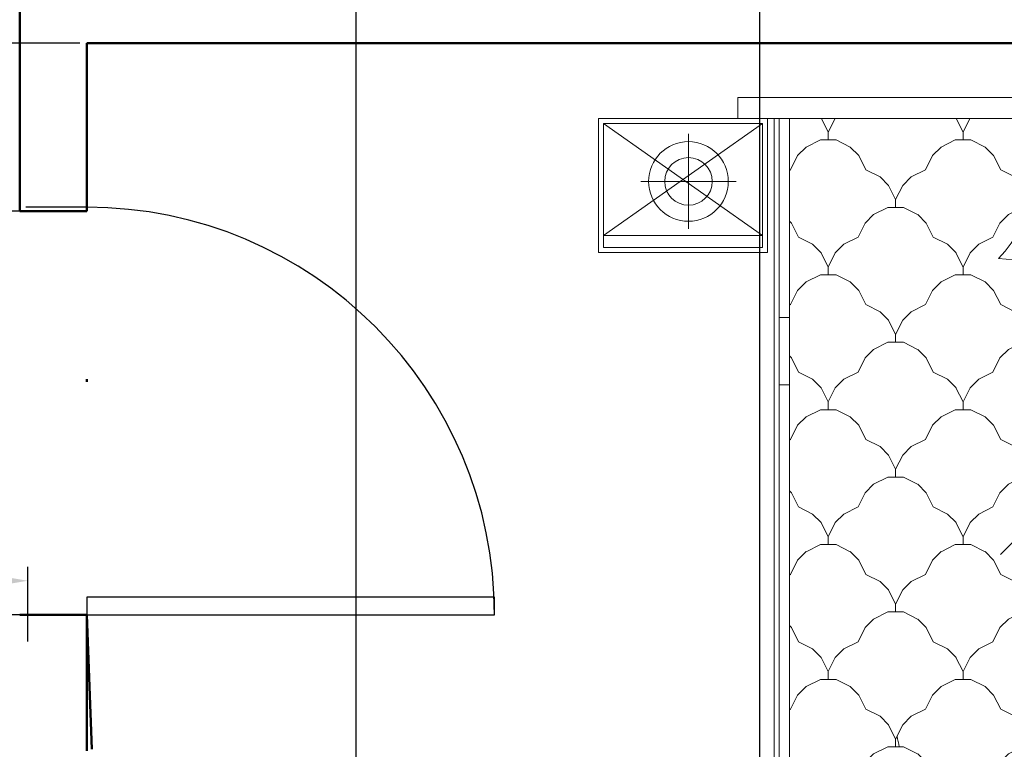
# Model space of a CAD drawing. Units: inches. Extents: x 2385 to 2740, y 1752 to 2305.
# Tile 4 of 15: x 2553 to 2641, y 1916 to 1981. Entities that reach past the tile are written whole.
import ezdxf

# ---------------------------------------------------------------- set-up
doc = ezdxf.new("R2010")
doc.units = ezdxf.units.IN
for name, color, linetype, lineweight in [('A-ANNO-DIMS', 2, 'Continuous', 18), ('A-DOOR', 4, 'Continuous', 25), ('A-FURN', 9, 'Continuous', 18), ('A-WALL', 7, 'Continuous', 50)]:
    doc.layers.add(name, color=color, linetype=linetype, lineweight=lineweight)
doc.styles.get("Standard").update_dxf_attribs({"font": 'arial.ttf'})
doc.dimstyles.new('Copy of ISO-25', dxfattribs={"dimtxt": 2.5, "dimasz": 2.5, "dimexe": 1.25, "dimexo": 0.625, "dimtad": 1, "dimdec": 1, "dimlunit": 4, "dimtxsty": 'Standard', "dimcen": 2.5, "dimadec": 0, "dimazin": 0, "dimtfac": 1, "dimtdec": 1, "dimtmove": 0, "dimatfit": 3, "dimfxl": 1, "dimarcsym": 0})

# ---------------------------------------------------------------- blocks, each defined once
blk = doc.blocks.new('A$C029D5C69')
for p, q in [((0.4164, 2.0693), (0.4164, 2.0066)), ((2.2315, 2.0693), (0.4164, 2.0693)), ((2.2315, 2.0066), (2.2315, 2.0693)), ((0, 1.606), (0, 2.0066)), ((0, 2.0066), (0.505, 2.0066)), ((0.4164, 2.0066), (2.2315, 2.0066)), ((0.505, 2.0066), (0.505, 1.606)), ((0.5252, 0.0351), (0.5252, 2.0066)), ((0.5403, 0.0502), (0.5403, 2.0066)), ((0.5706, 0.0805), (0.5706, 2.0066)), ((0.6869, 1.966), (0.6666, 2.0066)), ((0.7072, 2.0066), (0.6869, 1.966)), ((1.0902, 1.966), (1.0699, 2.0066)), ((1.1106, 2.0066), (1.0902, 1.966)), ((2.1114, 2.0087), (2.1114, 0.0351)), ((2.6479, 2.0066), (2.1429, 2.0066)), ((2.1429, 2.0066), (2.1429, 1.606)), ((2.6479, 1.606), (2.6479, 2.0066)), ((0.0151, 1.6211), (0.0151, 1.9915)), ((0.0151, 1.9915), (0.4899, 1.9915)), ((0.4899, 1.9915), (0.4899, 1.6211)), ((1.8954, 1.9865), (1.3081, 1.9865)), ((2.6328, 1.9915), (2.158, 1.9915)), ((2.158, 1.9915), (2.158, 1.6211)), ((2.6328, 1.6211), (2.6328, 1.9915)), ((0.2689, 1.9609), (0.2689, 1.6764)), ((0.6869, 1.9425), (0.6869, 1.966)), ((0.6869, 1.9425), (0.6869, 1.966)), ((1.0902, 1.9425), (1.0902, 1.966)), ((1.0902, 1.9425), (1.0902, 1.966)), ((1.8954, 1.9713), (1.3339, 1.9713)), ((1.3849, 1.9713), (1.3656, 1.952)), ((1.3945, 1.9713), (1.3714, 1.9483)), ((1.4249, 1.945), (1.3986, 1.9713)), ((1.4249, 1.945), (1.4059, 1.926)), ((1.4288, 1.9507), (1.4081, 1.9713)), ((1.4476, 1.9507), (1.4288, 1.9507)), ((1.4476, 1.9507), (1.4664, 1.9507)), ((1.487, 1.9713), (1.4664, 1.9507)), ((1.4966, 1.9713), (1.4703, 1.945)), ((1.4986, 1.9167), (1.4703, 1.945)), ((1.527, 1.945), (1.4986, 1.9167)), ((1.527, 1.945), (1.5007, 1.9713)), ((1.5309, 1.9507), (1.5102, 1.9713)), ((1.5497, 1.9507), (1.5309, 1.9507)), ((1.5497, 1.9507), (1.5685, 1.9507)), ((1.5891, 1.9713), (1.5685, 1.9507)), ((1.5987, 1.9713), (1.5724, 1.945)), ((1.6007, 1.9167), (1.5724, 1.945)), ((1.6291, 1.945), (1.6007, 1.9167)), ((1.6291, 1.945), (1.6028, 1.9713)), ((1.633, 1.9507), (1.6123, 1.9713)), ((1.6518, 1.9507), (1.633, 1.9507)), ((1.6518, 1.9507), (1.6706, 1.9507)), ((1.6912, 1.9713), (1.6706, 1.9507)), ((1.7008, 1.9713), (1.6745, 1.945)), ((1.7028, 1.9167), (1.6745, 1.945)), ((1.7312, 1.945), (1.7028, 1.9167)), ((1.7312, 1.945), (1.7049, 1.9713)), ((1.7351, 1.9507), (1.7144, 1.9713)), ((1.7539, 1.9507), (1.7351, 1.9507)), ((1.7539, 1.9507), (1.7727, 1.9507)), ((1.7933, 1.9713), (1.7727, 1.9507)), ((1.8029, 1.9713), (1.7766, 1.945)), ((1.8049, 1.9167), (1.7766, 1.945)), ((1.8333, 1.945), (1.8049, 1.9167)), ((1.8333, 1.945), (1.807, 1.9713)), ((1.8372, 1.9507), (1.8165, 1.9713)), ((1.856, 1.9507), (1.8372, 1.9507)), ((1.856, 1.9507), (1.8748, 1.9507)), ((1.8954, 1.9713), (1.8748, 1.9507)), ((1.9043, 1.9707), (1.8787, 1.945)), ((1.907, 1.9167), (1.8787, 1.945)), ((1.9354, 1.945), (1.907, 1.9167)), ((1.9354, 1.945), (1.9114, 1.969)), ((2.379, 1.9609), (2.379, 1.6764)), ((0.621, 1.9213), (0.5955, 1.8958)), ((0.6634, 1.9425), (0.621, 1.9213)), ((0.6634, 1.9425), (0.621, 1.9213)), ((0.6869, 1.9425), (0.6634, 1.9425)), ((0.6869, 1.9425), (0.7104, 1.9425)), ((0.7528, 1.9213), (0.7104, 1.9425)), ((0.7528, 1.9213), (0.7104, 1.9425)), ((0.7783, 1.8958), (0.7528, 1.9213)), ((1.0243, 1.9213), (0.9988, 1.8958)), ((1.0668, 1.9425), (1.0244, 1.9213)), ((1.0668, 1.9425), (1.0244, 1.9213)), ((1.0902, 1.9425), (1.0668, 1.9425)), ((1.0902, 1.9425), (1.1137, 1.9425)), ((1.1561, 1.9213), (1.1137, 1.9425)), ((1.1561, 1.9213), (1.1137, 1.9425)), ((1.1816, 1.8958), (1.1561, 1.9213)), ((1.4288, 1.9394), (1.4116, 1.9222)), ((1.4288, 1.9393), (1.4476, 1.9393)), ((1.4664, 1.9393), (1.4476, 1.9393)), ((1.493, 1.9128), (1.4664, 1.9394)), ((1.5309, 1.9394), (1.5043, 1.9128)), ((1.5309, 1.9393), (1.5497, 1.9393)), ((1.5685, 1.9393), (1.5497, 1.9393)), ((1.595, 1.9128), (1.5685, 1.9394)), ((1.633, 1.9394), (1.6064, 1.9128)), ((1.633, 1.9393), (1.6518, 1.9393)), ((1.6706, 1.9393), (1.6518, 1.9393)), ((1.6971, 1.9128), (1.6706, 1.9394)), ((1.7351, 1.9394), (1.7085, 1.9128)), ((1.7351, 1.9393), (1.7539, 1.9393)), ((1.7727, 1.9393), (1.7539, 1.9393)), ((1.7992, 1.9128), (1.7727, 1.9394)), ((1.8372, 1.9394), (1.8106, 1.9128)), ((1.8372, 1.9393), (1.856, 1.9393)), ((1.8748, 1.9393), (1.856, 1.9393)), ((1.9013, 1.9128), (1.8748, 1.9394)), ((1.9393, 1.9394), (1.9127, 1.9128)), ((1.9393, 1.9393), (1.9404, 1.9393)), ((1.9414, 1.688), (1.9414, 1.931)), ((1.9565, 1.688), (1.9565, 1.931)), ((0.5955, 1.8958), (0.5743, 1.8534)), ((0.7995, 1.8534), (0.7783, 1.8958)), ((0.9989, 1.8958), (0.9777, 1.8534)), ((1.2028, 1.8534), (1.1816, 1.8958)), ((1.493, 1.8752), (1.493, 1.9128)), ((1.5043, 1.8752), (1.5043, 1.9128)), ((1.595, 1.8752), (1.595, 1.9128)), ((1.6064, 1.8752), (1.6064, 1.9128)), ((1.6971, 1.8752), (1.6971, 1.9128)), ((1.7085, 1.8752), (1.7085, 1.9128)), ((1.7992, 1.8752), (1.7992, 1.9128)), ((1.8106, 1.8752), (1.8106, 1.9128)), ((1.9013, 1.8752), (1.9013, 1.9128)), ((1.9127, 1.8752), (1.9127, 1.9128)), ((1.493, 1.8752), (1.4867, 1.869)), ((1.4986, 1.8713), (1.4922, 1.8648)), ((1.527, 1.8429), (1.4986, 1.8713)), ((1.5309, 1.8486), (1.5043, 1.8752)), ((1.595, 1.8752), (1.5685, 1.8486)), ((1.6007, 1.8713), (1.5724, 1.8429)), ((1.6291, 1.8429), (1.6007, 1.8713)), ((1.633, 1.8486), (1.6064, 1.8752)), ((1.6971, 1.8752), (1.6706, 1.8486)), ((1.7028, 1.8713), (1.6745, 1.8429)), ((1.7312, 1.8429), (1.7028, 1.8713)), ((1.7351, 1.8486), (1.7085, 1.8752)), ((1.7992, 1.8752), (1.7727, 1.8486)), ((1.8049, 1.8713), (1.7766, 1.8429)), ((1.8333, 1.8429), (1.8049, 1.8713)), ((1.8372, 1.8486), (1.8106, 1.8752)), ((1.9013, 1.8752), (1.8748, 1.8486)), ((1.907, 1.8713), (1.8787, 1.8429)), ((1.9354, 1.8429), (1.907, 1.8713)), ((1.9393, 1.8486), (1.9127, 1.8752)), ((0.5743, 1.8534), (0.5706, 1.8515)), ((0.5743, 1.8534), (0.5706, 1.8515)), ((0.8419, 1.8322), (0.7995, 1.8534)), ((0.8419, 1.8322), (0.7995, 1.8534)), ((0.8674, 1.8067), (0.8419, 1.8322)), ((0.9352, 1.8322), (0.9097, 1.8067)), ((0.9777, 1.8534), (0.9353, 1.8322)), ((0.9777, 1.8534), (0.9353, 1.8322)), ((1.2452, 1.8322), (1.2028, 1.8534)), ((1.2452, 1.8322), (1.2028, 1.8534)), ((1.2707, 1.8067), (1.2452, 1.8322)), ((1.527, 1.8429), (1.5242, 1.8401)), ((1.5309, 1.8373), (1.5295, 1.8359)), ((1.5497, 1.8486), (1.5309, 1.8486)), ((1.5309, 1.8373), (1.5497, 1.8373)), ((1.5497, 1.8486), (1.5685, 1.8486)), ((1.5685, 1.8373), (1.5497, 1.8373)), ((1.595, 1.8107), (1.5685, 1.8373)), ((1.6007, 1.8146), (1.5724, 1.8429)), ((1.6291, 1.8429), (1.6007, 1.8146)), ((1.633, 1.8373), (1.6064, 1.8107)), ((1.6518, 1.8486), (1.633, 1.8486)), ((1.633, 1.8373), (1.6518, 1.8373)), ((1.6518, 1.8486), (1.6706, 1.8486)), ((1.6706, 1.8373), (1.6518, 1.8373)), ((1.6971, 1.8107), (1.6706, 1.8373)), ((1.7028, 1.8146), (1.6745, 1.8429)), ((1.7312, 1.8429), (1.7028, 1.8146)), ((1.7351, 1.8373), (1.7085, 1.8107)), ((1.7539, 1.8486), (1.7351, 1.8486)), ((1.7351, 1.8373), (1.7539, 1.8373)), ((1.7539, 1.8486), (1.7727, 1.8486)), ((1.7727, 1.8373), (1.7539, 1.8373)), ((1.7992, 1.8107), (1.7727, 1.8373)), ((1.8049, 1.8146), (1.7766, 1.8429)), ((1.8333, 1.8429), (1.8049, 1.8146)), ((1.8372, 1.8373), (1.8106, 1.8107)), ((1.856, 1.8486), (1.8372, 1.8486)), ((1.8372, 1.8373), (1.856, 1.8373)), ((1.856, 1.8486), (1.8748, 1.8486)), ((1.8748, 1.8373), (1.856, 1.8373)), ((1.9013, 1.8107), (1.8748, 1.8373)), ((1.907, 1.8146), (1.8787, 1.8429)), ((1.9354, 1.8429), (1.907, 1.8146)), ((1.9393, 1.8373), (1.9127, 1.8107)), ((1.9414, 1.8486), (1.9393, 1.8486)), ((1.9393, 1.8373), (1.9414, 1.8373)), ((0.1267, 1.8186), (0.4111, 1.8186)), ((0.8886, 1.7643), (0.8674, 1.8067)), ((0.9098, 1.8067), (0.8886, 1.7643)), ((1.2919, 1.7643), (1.2707, 1.8067)), ((1.595, 1.7806), (1.595, 1.8107)), ((1.6064, 1.7731), (1.6064, 1.8107)), ((1.6971, 1.7731), (1.6971, 1.8107)), ((1.7085, 1.7731), (1.7085, 1.8107)), ((1.7992, 1.7731), (1.7992, 1.8107)), ((1.8106, 1.7731), (1.8106, 1.8107)), ((1.9013, 1.7731), (1.9013, 1.8107)), ((1.9127, 1.7731), (1.9127, 1.8107)), ((2.2367, 1.8186), (2.5212, 1.8186)), ((1.2981, 1.7768), (1.2919, 1.7643)), ((1.633, 1.7465), (1.6064, 1.7731)), ((1.6971, 1.7731), (1.6706, 1.7465)), ((1.7028, 1.7692), (1.6745, 1.7408)), ((1.7312, 1.7408), (1.7028, 1.7692)), ((1.7351, 1.7465), (1.7085, 1.7731)), ((1.7992, 1.7731), (1.7727, 1.7465)), ((1.8049, 1.7692), (1.7766, 1.7408)), ((1.8333, 1.7408), (1.8049, 1.7692)), ((1.8372, 1.7465), (1.8106, 1.7731)), ((1.9013, 1.7731), (1.8748, 1.7465)), ((1.907, 1.7692), (1.8787, 1.7408)), ((1.9354, 1.7408), (1.907, 1.7692)), ((1.9393, 1.7465), (1.9127, 1.7731)), ((0.8651, 1.7408), (0.8227, 1.7196)), ((0.8651, 1.7408), (0.8227, 1.7196)), ((0.912, 1.7408), (0.8651, 1.7408)), ((0.8886, 1.7408), (0.8886, 1.7643)), ((0.9544, 1.7196), (0.912, 1.7408)), ((0.9544, 1.7196), (0.912, 1.7408)), ((1.2684, 1.7408), (1.226, 1.7196)), ((1.2684, 1.7408), (1.226, 1.7196)), ((1.2885, 1.7408), (1.2684, 1.7408)), ((1.2919, 1.7519), (1.2919, 1.7643)), ((1.6518, 1.7465), (1.633, 1.7465)), ((1.6518, 1.7465), (1.6706, 1.7465)), ((1.7028, 1.7125), (1.6745, 1.7408)), ((1.7312, 1.7408), (1.7028, 1.7125)), ((1.7539, 1.7465), (1.7351, 1.7465)), ((1.7539, 1.7465), (1.7727, 1.7465)), ((1.8049, 1.7125), (1.7766, 1.7408)), ((1.8333, 1.7408), (1.8049, 1.7125)), ((1.856, 1.7465), (1.8372, 1.7465)), ((1.856, 1.7465), (1.8748, 1.7465)), ((1.907, 1.7125), (1.8787, 1.7408)), ((1.9354, 1.7408), (1.907, 1.7125)), ((1.9414, 1.7465), (1.9393, 1.7465)), ((0.8227, 1.7196), (0.7972, 1.6941)), ((0.98, 1.6941), (0.9545, 1.7196)), ((1.226, 1.7196), (1.2005, 1.6941)), ((1.6443, 1.7352), (1.6518, 1.7352)), ((1.6706, 1.7352), (1.6518, 1.7352)), ((1.6971, 1.7086), (1.6706, 1.7352)), ((1.6971, 1.682), (1.6971, 1.7086)), ((1.7351, 1.7352), (1.7085, 1.7086)), ((1.7085, 1.671), (1.7085, 1.7086)), ((1.7351, 1.7352), (1.7539, 1.7352)), ((1.7727, 1.7352), (1.7539, 1.7352)), ((1.7992, 1.7086), (1.7727, 1.7352)), ((1.7992, 1.671), (1.7992, 1.7086)), ((1.8372, 1.7352), (1.8106, 1.7086)), ((1.8106, 1.671), (1.8106, 1.7086)), ((1.8372, 1.7352), (1.856, 1.7352)), ((1.8748, 1.7352), (1.856, 1.7352)), ((1.9013, 1.7086), (1.8748, 1.7352)), ((1.9013, 1.671), (1.9013, 1.7086)), ((1.9393, 1.7352), (1.9127, 1.7086)), ((1.9127, 1.671), (1.9127, 1.7086)), ((1.9393, 1.7352), (1.9414, 1.7352)), ((0.5766, 1.6941), (0.5706, 1.7002)), ((0.5978, 1.6517), (0.5766, 1.6941)), ((0.7972, 1.6941), (0.776, 1.6517)), ((1.0011, 1.6517), (0.9799, 1.6941)), ((1.2005, 1.6941), (1.1793, 1.6517)), ((2.5551, 1.6275), (2.5551, 1.696)), ((0.6402, 1.6305), (0.5978, 1.6517)), ((0.6402, 1.6305), (0.5978, 1.6517)), ((0.776, 1.6517), (0.7336, 1.6305)), ((0.776, 1.6517), (0.7336, 1.6305)), ((1.0435, 1.6305), (1.0011, 1.6517)), ((1.0435, 1.6305), (1.0011, 1.6517)), ((1.1793, 1.6517), (1.1369, 1.6305)), ((1.1793, 1.6517), (1.1369, 1.6305)), ((1.7318, 1.6477), (1.7085, 1.671)), ((1.7992, 1.671), (1.7759, 1.6477)), ((1.8049, 1.6671), (1.7855, 1.6477)), ((1.8244, 1.6477), (1.8049, 1.6671)), ((1.8339, 1.6477), (1.8106, 1.671)), ((1.9013, 1.671), (1.878, 1.6477)), ((1.907, 1.6671), (1.8876, 1.6477)), ((1.9202, 1.6539), (1.907, 1.6671)), ((1.926, 1.6577), (1.9127, 1.671)), ((0.4899, 1.6211), (0.0151, 1.6211)), ((0.6657, 1.605), (0.6402, 1.6305)), ((0.7336, 1.6305), (0.7081, 1.605)), ((1.0691, 1.605), (1.0436, 1.6305)), ((1.1369, 1.6305), (1.1114, 1.605)), ((1.8961, 1.6477), (1.7289, 1.6477)), ((1.8961, 1.6325), (1.7422, 1.6325)), ((2.158, 1.6211), (2.6328, 1.6211)), ((0.505, 1.606), (0, 1.606)), ((0.6869, 1.5626), (0.6657, 1.605)), ((0.7081, 1.605), (0.6869, 1.5626)), ((1.0902, 1.5626), (1.069, 1.605)), ((1.1114, 1.605), (1.0902, 1.5626)), ((2.1429, 1.606), (2.6479, 1.606)), ((0.6869, 1.5392), (0.6869, 1.5626)), ((0.6869, 1.5392), (0.6869, 1.5626)), ((1.0902, 1.5392), (1.0902, 1.5626)), ((1.0902, 1.5392), (1.0902, 1.5626)), ((0.6634, 1.5391), (0.621, 1.5179)), ((0.6634, 1.5391), (0.621, 1.5179)), ((0.6869, 1.5392), (0.6634, 1.5392)), ((0.6869, 1.5392), (0.7104, 1.5392)), ((0.7528, 1.5179), (0.7104, 1.5391)), ((0.7528, 1.5179), (0.7104, 1.5391)), ((1.0668, 1.5391), (1.0244, 1.5179)), ((1.0668, 1.5391), (1.0244, 1.5179)), ((1.0902, 1.5392), (1.0668, 1.5392)), ((1.0902, 1.5392), (1.1137, 1.5392)), ((1.1561, 1.5179), (1.1137, 1.5391)), ((1.1561, 1.5179), (1.1137, 1.5391)), ((0.621, 1.5179), (0.5955, 1.4924)), ((0.7783, 1.4924), (0.7528, 1.5179)), ((1.0243, 1.5179), (0.9988, 1.4924)), ((1.1816, 1.4924), (1.1561, 1.5179)), ((1.4277, 1.5179), (1.4022, 1.4924)), ((1.4534, 1.5308), (1.4277, 1.5179)), ((1.4534, 1.5308), (1.4277, 1.5179)), ((0.5955, 1.4925), (0.5743, 1.4501)), ((0.7995, 1.4501), (0.7783, 1.4925)), ((0.9989, 1.4925), (0.9777, 1.4501)), ((1.2028, 1.4501), (1.1816, 1.4925)), ((1.4022, 1.4925), (1.381, 1.4501)), ((0.5743, 1.45), (0.5706, 1.4481)), ((0.5743, 1.45), (0.5706, 1.4481)), ((0.8419, 1.4288), (0.7995, 1.45)), ((0.8419, 1.4288), (0.7995, 1.45)), ((0.9777, 1.45), (0.9353, 1.4288)), ((0.9777, 1.45), (0.9353, 1.4288)), ((1.2452, 1.4288), (1.2028, 1.45)), ((1.2452, 1.4288), (1.2028, 1.45)), ((1.381, 1.45), (1.3386, 1.4288)), ((1.381, 1.45), (1.3386, 1.4288)), ((1.6062, 1.4501), (1.5966, 1.4692)), ((1.6486, 1.4288), (1.6062, 1.45)), ((1.6486, 1.4288), (1.6062, 1.45)), ((0.8674, 1.4033), (0.8419, 1.4288)), ((0.9352, 1.4288), (0.9097, 1.4033)), ((1.2707, 1.4033), (1.2452, 1.4288)), ((1.3386, 1.4288), (1.3131, 1.4033)), ((1.6741, 1.4033), (1.6486, 1.4288)), ((0.5403, 1.4117), (0.5706, 1.4117)), ((0.8886, 1.361), (0.8674, 1.4034)), ((0.9098, 1.4034), (0.8886, 1.361)), ((1.2919, 1.361), (1.2707, 1.4034)), ((1.3131, 1.4034), (1.2919, 1.361)), ((1.6953, 1.361), (1.6741, 1.4034)), ((1.714, 1.3984), (1.6953, 1.361)), ((0.8886, 1.3375), (0.8886, 1.3609)), ((1.2919, 1.3375), (1.2919, 1.3609)), ((1.6953, 1.3375), (1.6953, 1.3609)), ((0.8651, 1.3374), (0.8227, 1.3162)), ((0.8651, 1.3374), (0.8227, 1.3162)), ((0.912, 1.3375), (0.8651, 1.3375)), ((0.9544, 1.3162), (0.912, 1.3374)), ((0.9544, 1.3162), (0.912, 1.3374)), ((1.2684, 1.3374), (1.226, 1.3162)), ((1.2684, 1.3374), (1.226, 1.3162)), ((1.3154, 1.3375), (1.2684, 1.3375)), ((1.3578, 1.3162), (1.3154, 1.3374)), ((1.3578, 1.3162), (1.3154, 1.3374)), ((1.6718, 1.3374), (1.6294, 1.3162)), ((1.6718, 1.3374), (1.6294, 1.3162)), ((1.7187, 1.3375), (1.6718, 1.3375)), ((1.7611, 1.3162), (1.7187, 1.3374)), ((1.7611, 1.3162), (1.7187, 1.3374)), ((0.5766, 1.2908), (0.5706, 1.2968)), ((0.8227, 1.3163), (0.7972, 1.2908)), ((0.98, 1.2908), (0.9545, 1.3163)), ((1.226, 1.3163), (1.2005, 1.2908)), ((1.3833, 1.2908), (1.3578, 1.3163)), ((1.6294, 1.3163), (1.6039, 1.2908)), ((1.7867, 1.2908), (1.7611, 1.3163)), ((0.5978, 1.2484), (0.5766, 1.2908)), ((0.7972, 1.2908), (0.776, 1.2484)), ((1.0011, 1.2484), (0.9799, 1.2908)), ((1.2005, 1.2908), (1.1793, 1.2484)), ((1.4045, 1.2484), (1.3833, 1.2908)), ((1.6039, 1.2908), (1.5827, 1.2484)), ((1.8078, 1.2484), (1.7866, 1.2908)), ((0.6402, 1.2271), (0.5978, 1.2483)), ((0.6402, 1.2271), (0.5978, 1.2483)), ((0.776, 1.2483), (0.7336, 1.2271)), ((0.776, 1.2483), (0.7336, 1.2271)), ((1.0435, 1.2271), (1.0011, 1.2483)), ((1.0435, 1.2271), (1.0011, 1.2483)), ((1.1793, 1.2483), (1.1369, 1.2271)), ((1.1793, 1.2483), (1.1369, 1.2271)), ((1.4469, 1.2271), (1.4045, 1.2483)), ((1.4469, 1.2271), (1.4045, 1.2483)), ((1.5827, 1.2483), (1.5403, 1.2271)), ((1.5827, 1.2483), (1.5403, 1.2271)), ((1.8502, 1.2271), (1.8078, 1.2483)), ((1.8502, 1.2271), (1.8078, 1.2483)), ((0.5403, 1.21), (0.5706, 1.21)), ((0.6657, 1.2017), (0.6402, 1.2272)), ((0.7336, 1.2272), (0.7081, 1.2017)), ((1.0691, 1.2017), (1.0436, 1.2272)), ((1.1369, 1.2272), (1.1114, 1.2017)), ((1.4724, 1.2017), (1.4469, 1.2272)), ((1.5403, 1.2272), (1.5148, 1.2017)), ((1.8758, 1.2017), (1.8503, 1.2272)), ((0.6869, 1.1593), (0.6657, 1.2017)), ((0.7081, 1.2017), (0.6869, 1.1593)), ((1.0902, 1.1593), (1.069, 1.2017)), ((1.1114, 1.2017), (1.0902, 1.1593)), ((1.4936, 1.1593), (1.4724, 1.2017)), ((1.5148, 1.2017), (1.4936, 1.1593)), ((1.8969, 1.1593), (1.8757, 1.2017)), ((1.9181, 1.2017), (1.8969, 1.1593)), ((1.9215, 1.2051), (1.9181, 1.2017)), ((0.6869, 1.1358), (0.6869, 1.1593)), ((0.6869, 1.1358), (0.6869, 1.1593)), ((1.0902, 1.1358), (1.0902, 1.1593)), ((1.0902, 1.1358), (1.0902, 1.1593)), ((1.4936, 1.1358), (1.4936, 1.1593)), ((1.4936, 1.1358), (1.4936, 1.1593)), ((1.8969, 1.1358), (1.8969, 1.1593)), ((1.8969, 1.1358), (1.8969, 1.1593)), ((0.6634, 1.1358), (0.621, 1.1146)), ((0.6634, 1.1358), (0.621, 1.1146)), ((0.6869, 1.1358), (0.6634, 1.1358)), ((0.6869, 1.1358), (0.7104, 1.1358)), ((0.7528, 1.1146), (0.7104, 1.1358)), ((0.7528, 1.1146), (0.7104, 1.1358)), ((1.0668, 1.1358), (1.0244, 1.1146)), ((1.0668, 1.1358), (1.0244, 1.1146)), ((1.0902, 1.1358), (1.0668, 1.1358)), ((1.0902, 1.1358), (1.1137, 1.1358)), ((1.1561, 1.1146), (1.1137, 1.1358)), ((1.1561, 1.1146), (1.1137, 1.1358)), ((1.4701, 1.1358), (1.4277, 1.1146)), ((1.4701, 1.1358), (1.4277, 1.1146)), ((1.4936, 1.1358), (1.4701, 1.1358)), ((1.4936, 1.1358), (1.5171, 1.1358)), ((1.5595, 1.1146), (1.5171, 1.1358)), ((1.5595, 1.1146), (1.5171, 1.1358)), ((1.8735, 1.1358), (1.8311, 1.1146)), ((1.8735, 1.1358), (1.8311, 1.1146)), ((1.8969, 1.1358), (1.8735, 1.1358)), ((1.8969, 1.1358), (1.9204, 1.1358)), ((1.9628, 1.1146), (1.9204, 1.1358)), ((1.9628, 1.1146), (1.9204, 1.1358)), ((0.621, 1.1146), (0.5955, 1.0891)), ((0.7783, 1.0891), (0.7528, 1.1146)), ((1.0243, 1.1146), (0.9988, 1.0891)), ((1.1816, 1.0891), (1.1561, 1.1146)), ((1.4277, 1.1146), (1.4022, 1.0891)), ((1.585, 1.0891), (1.5595, 1.1146)), ((1.831, 1.1146), (1.8055, 1.0891)), ((1.9883, 1.0891), (1.9628, 1.1146)), ((0.5955, 1.0891), (0.5743, 1.0467)), ((0.7995, 1.0467), (0.7783, 1.0891)), ((0.9989, 1.0891), (0.9777, 1.0467)), ((1.2028, 1.0467), (1.1816, 1.0891)), ((1.4022, 1.0891), (1.381, 1.0467)), ((1.6062, 1.0467), (1.585, 1.0891)), ((1.8056, 1.0891), (1.7844, 1.0467)), ((2.0095, 1.0467), (1.9883, 1.0891)), ((0.5743, 1.0467), (0.5706, 1.0448)), ((0.5743, 1.0467), (0.5706, 1.0448)), ((0.8419, 1.0255), (0.7995, 1.0467)), ((0.8419, 1.0255), (0.7995, 1.0467)), ((0.9777, 1.0467), (0.9353, 1.0255)), ((0.9777, 1.0467), (0.9353, 1.0255)), ((1.2452, 1.0255), (1.2028, 1.0467)), ((1.2452, 1.0255), (1.2028, 1.0467)), ((1.381, 1.0467), (1.3386, 1.0255)), ((1.381, 1.0467), (1.3386, 1.0255)), ((1.6486, 1.0255), (1.6062, 1.0467)), ((1.6486, 1.0255), (1.6062, 1.0467)), ((1.7844, 1.0467), (1.742, 1.0255)), ((1.7844, 1.0467), (1.742, 1.0255)), ((2.0276, 1.0376), (2.0095, 1.0467)), ((2.0276, 1.0376), (2.0095, 1.0467)), ((0.8674, 1), (0.8419, 1.0255)), ((0.9352, 1.0255), (0.9097, 1)), ((1.2707, 1), (1.2452, 1.0255)), ((1.3386, 1.0255), (1.3131, 1)), ((1.6741, 1), (1.6486, 1.0255)), ((1.7419, 1.0255), (1.7164, 1)), ((0.8886, 0.9576), (0.8674, 1)), ((0.9098, 1), (0.8886, 0.9576)), ((1.2919, 0.9576), (1.2707, 1)), ((1.3131, 1), (1.2919, 0.9576)), ((1.6953, 0.9576), (1.6741, 1)), ((1.7165, 1), (1.6953, 0.9576)), ((0.8886, 0.9341), (0.8886, 0.9576)), ((1.2919, 0.9341), (1.2919, 0.9576)), ((1.6953, 0.9341), (1.6953, 0.9576)), ((2.066, 0.9457), (2.066, 0.0805)), ((0.8651, 0.9341), (0.8227, 0.9129)), ((0.8651, 0.9341), (0.8227, 0.9129)), ((0.912, 0.9341), (0.8651, 0.9341)), ((0.9544, 0.9129), (0.912, 0.9341)), ((0.9544, 0.9129), (0.912, 0.9341)), ((1.2684, 0.9341), (1.226, 0.9129)), ((1.2684, 0.9341), (1.226, 0.9129)), ((1.3154, 0.9341), (1.2684, 0.9341)), ((1.3578, 0.9129), (1.3154, 0.9341)), ((1.3578, 0.9129), (1.3154, 0.9341)), ((1.6718, 0.9341), (1.6294, 0.9129)), ((1.6718, 0.9341), (1.6294, 0.9129)), ((1.7187, 0.9341), (1.6718, 0.9341)), ((1.7611, 0.9129), (1.7187, 0.9341)), ((1.7611, 0.9129), (1.7187, 0.9341)), ((2.066, 0.9295), (2.0327, 0.9129)), ((2.066, 0.9295), (2.0327, 0.9129)), ((0.5766, 0.8874), (0.5706, 0.8935)), ((0.5978, 0.845), (0.5766, 0.8874)), ((0.7972, 0.8874), (0.776, 0.845)), ((0.8227, 0.9129), (0.7972, 0.8874)), ((0.98, 0.8874), (0.9545, 0.9129)), ((1.0011, 0.845), (0.9799, 0.8874)), ((1.2005, 0.8874), (1.1793, 0.845)), ((1.226, 0.9129), (1.2005, 0.8874)), ((1.3833, 0.8874), (1.3578, 0.9129)), ((1.4045, 0.845), (1.3833, 0.8874)), ((1.6039, 0.8874), (1.5827, 0.845)), ((1.6294, 0.9129), (1.6039, 0.8874)), ((1.7867, 0.8874), (1.7611, 0.9129)), ((1.8078, 0.845), (1.7866, 0.8874)), ((2.0072, 0.8874), (1.986, 0.845)), ((2.0327, 0.9129), (2.0072, 0.8874)), ((0.6402, 0.8238), (0.5978, 0.845)), ((0.6402, 0.8238), (0.5978, 0.845)), ((0.776, 0.845), (0.7336, 0.8238)), ((0.776, 0.845), (0.7336, 0.8238)), ((1.0435, 0.8238), (1.0011, 0.845)), ((1.0435, 0.8238), (1.0011, 0.845)), ((1.1793, 0.845), (1.1369, 0.8238)), ((1.1793, 0.845), (1.1369, 0.8238)), ((1.4469, 0.8238), (1.4045, 0.845)), ((1.4469, 0.8238), (1.4045, 0.845)), ((1.5827, 0.845), (1.5403, 0.8238)), ((1.5827, 0.845), (1.5403, 0.8238)), ((1.8502, 0.8238), (1.8078, 0.845)), ((1.8502, 0.8238), (1.8078, 0.845)), ((1.986, 0.845), (1.9436, 0.8238)), ((1.986, 0.845), (1.9436, 0.8238)), ((2.0962, 0.8369), (2.0962, 0.0502)), ((0.6657, 0.7983), (0.6402, 0.8238)), ((0.6869, 0.7559), (0.6657, 0.7983)), ((0.7081, 0.7983), (0.6869, 0.7559)), ((0.7336, 0.8238), (0.7081, 0.7983)), ((1.0691, 0.7983), (1.0436, 0.8238)), ((1.0902, 0.7559), (1.069, 0.7983)), ((1.1114, 0.7983), (1.0902, 0.7559)), ((1.1369, 0.8238), (1.1114, 0.7983)), ((1.4724, 0.7983), (1.4469, 0.8238)), ((1.4936, 0.7559), (1.4724, 0.7983)), ((1.5148, 0.7983), (1.4936, 0.7559)), ((1.5403, 0.8238), (1.5148, 0.7983)), ((1.8758, 0.7983), (1.8503, 0.8238)), ((1.8969, 0.7559), (1.8757, 0.7983)), ((1.9181, 0.7983), (1.8969, 0.7559)), ((1.9436, 0.8238), (1.9181, 0.7983)), ((0.6869, 0.7325), (0.6869, 0.7559)), ((0.6869, 0.7325), (0.6869, 0.7559)), ((1.0902, 0.7325), (1.0902, 0.7559)), ((1.0902, 0.7325), (1.0902, 0.7559)), ((1.2024, 0.7028), (1.2503, 0.7507)), ((1.4936, 0.7325), (1.4936, 0.7559)), ((1.4936, 0.7325), (1.4936, 0.7559)), ((1.8969, 0.7325), (1.8969, 0.7559)), ((1.8969, 0.7325), (1.8969, 0.7559)), ((0.621, 0.7113), (0.5955, 0.6858)), ((0.6634, 0.7324), (0.621, 0.7112)), ((0.6634, 0.7324), (0.621, 0.7112)), ((0.6869, 0.7325), (0.6634, 0.7325)), ((0.6869, 0.7325), (0.7104, 0.7325)), ((0.7528, 0.7112), (0.7104, 0.7324)), ((0.7528, 0.7112), (0.7104, 0.7324)), ((0.7783, 0.6858), (0.7528, 0.7113)), ((1.0243, 0.7113), (0.9988, 0.6858)), ((1.0668, 0.7324), (1.0244, 0.7112)), ((1.0668, 0.7324), (1.0244, 0.7112)), ((1.0902, 0.7325), (1.0668, 0.7325)), ((1.0902, 0.7325), (1.1137, 0.7325)), ((1.1561, 0.7112), (1.1137, 0.7324)), ((1.1561, 0.7112), (1.1137, 0.7324)), ((1.1816, 0.6858), (1.1561, 0.7113)), ((1.4277, 0.7113), (1.4022, 0.6858)), ((1.4701, 0.7324), (1.4277, 0.7112)), ((1.4701, 0.7324), (1.4277, 0.7112)), ((1.4936, 0.7325), (1.4701, 0.7325)), ((1.4936, 0.7325), (1.5171, 0.7325)), ((1.5595, 0.7112), (1.5171, 0.7324)), ((1.5595, 0.7112), (1.5171, 0.7324)), ((1.585, 0.6858), (1.5595, 0.7113)), ((1.831, 0.7113), (1.8055, 0.6858)), ((1.8735, 0.7324), (1.8311, 0.7112)), ((1.8735, 0.7324), (1.8311, 0.7112)), ((1.8969, 0.7325), (1.8735, 0.7325)), ((1.8969, 0.7325), (1.9204, 0.7325)), ((1.9628, 0.7112), (1.9204, 0.7324)), ((1.9628, 0.7112), (1.9204, 0.7324)), ((1.9883, 0.6858), (1.9628, 0.7113)), ((0.5955, 0.6858), (0.5743, 0.6434)), ((0.7995, 0.6434), (0.7783, 0.6858)), ((0.9989, 0.6858), (0.9777, 0.6434)), ((1.2028, 0.6434), (1.1816, 0.6858)), ((1.4022, 0.6858), (1.381, 0.6434)), ((1.6062, 0.6434), (1.585, 0.6858)), ((1.8056, 0.6858), (1.7844, 0.6434)), ((2.0095, 0.6434), (1.9883, 0.6858)), ((0.5743, 0.6433), (0.5706, 0.6414)), ((0.5743, 0.6433), (0.5706, 0.6414)), ((0.8419, 0.6221), (0.7995, 0.6433)), ((0.8419, 0.6221), (0.7995, 0.6433)), ((0.8674, 0.5967), (0.8419, 0.6222)), ((0.9352, 0.6222), (0.9097, 0.5967)), ((0.9777, 0.6433), (0.9353, 0.6221)), ((0.9777, 0.6433), (0.9353, 0.6221)), ((1.2452, 0.6221), (1.2028, 0.6433)), ((1.2452, 0.6221), (1.2028, 0.6433)), ((1.2707, 0.5967), (1.2452, 0.6222)), ((1.3386, 0.6222), (1.3131, 0.5967)), ((1.381, 0.6433), (1.3386, 0.6221)), ((1.381, 0.6433), (1.3386, 0.6221)), ((1.6486, 0.6221), (1.6062, 0.6433)), ((1.6486, 0.6221), (1.6062, 0.6433)), ((1.6741, 0.5967), (1.6486, 0.6222)), ((1.7419, 0.6222), (1.7164, 0.5967)), ((1.7844, 0.6433), (1.742, 0.6221)), ((1.7844, 0.6433), (1.742, 0.6221)), ((2.0519, 0.6221), (2.0095, 0.6433)), ((2.0519, 0.6221), (2.0095, 0.6433)), ((2.066, 0.6081), (2.0519, 0.6222)), ((0.8886, 0.5543), (0.8674, 0.5967)), ((0.9098, 0.5967), (0.8886, 0.5543)), ((1.2919, 0.5543), (1.2707, 0.5967)), ((1.3131, 0.5967), (1.2919, 0.5543)), ((1.6953, 0.5543), (1.6741, 0.5967)), ((1.7165, 0.5967), (1.6953, 0.5543)), ((0.8651, 0.5308), (0.8227, 0.5096)), ((0.8651, 0.5308), (0.8227, 0.5096)), ((0.912, 0.5308), (0.8651, 0.5308)), ((0.8886, 0.5308), (0.8886, 0.5543)), ((0.9544, 0.5096), (0.912, 0.5308)), ((0.9544, 0.5096), (0.912, 0.5308)), ((1.2684, 0.5308), (1.226, 0.5096)), ((1.2684, 0.5308), (1.226, 0.5096)), ((1.3154, 0.5308), (1.2684, 0.5308)), ((1.2919, 0.5308), (1.2919, 0.5543)), ((1.3578, 0.5096), (1.3154, 0.5308)), ((1.3578, 0.5096), (1.3154, 0.5308)), ((1.6718, 0.5308), (1.6294, 0.5096)), ((1.6718, 0.5308), (1.6294, 0.5096)), ((1.7187, 0.5308), (1.6718, 0.5308)), ((1.6953, 0.5308), (1.6953, 0.5543)), ((1.7611, 0.5096), (1.7187, 0.5308)), ((1.7611, 0.5096), (1.7187, 0.5308)), ((0.8227, 0.5096), (0.7972, 0.4841)), ((0.98, 0.4841), (0.9545, 0.5096)), ((1.226, 0.5096), (1.2005, 0.4841)), ((1.3833, 0.4841), (1.3578, 0.5096)), ((1.6294, 0.5096), (1.6039, 0.4841)), ((1.7867, 0.4841), (1.7611, 0.5096)), ((2.0327, 0.5096), (2.0072, 0.4841)), ((2.066, 0.5262), (2.0327, 0.5096)), ((2.066, 0.5262), (2.0327, 0.5096)), ((0.5766, 0.4841), (0.5706, 0.4901)), ((0.5978, 0.4417), (0.5766, 0.4841)), ((0.7972, 0.4841), (0.776, 0.4417)), ((1.0011, 0.4417), (0.9799, 0.4841)), ((1.2005, 0.4841), (1.1793, 0.4417)), ((1.4045, 0.4417), (1.3833, 0.4841)), ((1.6039, 0.4841), (1.5827, 0.4417)), ((1.8078, 0.4417), (1.7866, 0.4841)), ((2.0072, 0.4841), (1.986, 0.4417)), ((0.6402, 0.4205), (0.5978, 0.4417)), ((0.6402, 0.4205), (0.5978, 0.4417)), ((0.6657, 0.395), (0.6402, 0.4205)), ((0.7336, 0.4205), (0.7081, 0.395)), ((0.776, 0.4417), (0.7336, 0.4205)), ((0.776, 0.4417), (0.7336, 0.4205)), ((1.0435, 0.4205), (1.0011, 0.4417)), ((1.0435, 0.4205), (1.0011, 0.4417)), ((1.0691, 0.395), (1.0436, 0.4205)), ((1.1369, 0.4205), (1.1114, 0.395)), ((1.1793, 0.4417), (1.1369, 0.4205)), ((1.1793, 0.4417), (1.1369, 0.4205)), ((1.4469, 0.4205), (1.4045, 0.4417)), ((1.4469, 0.4205), (1.4045, 0.4417)), ((1.4724, 0.395), (1.4469, 0.4205)), ((1.5403, 0.4205), (1.5148, 0.395)), ((1.5827, 0.4417), (1.5403, 0.4205)), ((1.5827, 0.4417), (1.5403, 0.4205)), ((1.8502, 0.4205), (1.8078, 0.4417)), ((1.8502, 0.4205), (1.8078, 0.4417)), ((1.8758, 0.395), (1.8503, 0.4205)), ((1.9436, 0.4205), (1.9181, 0.395)), ((1.986, 0.4417), (1.9436, 0.4205)), ((1.986, 0.4417), (1.9436, 0.4205)), ((0.6869, 0.3526), (0.6657, 0.395)), ((0.7081, 0.395), (0.6869, 0.3526)), ((1.0902, 0.3526), (1.069, 0.395)), ((1.1114, 0.395), (1.0902, 0.3526)), ((1.4936, 0.3526), (1.4724, 0.395)), ((1.5148, 0.395), (1.4936, 0.3526)), ((1.8969, 0.3526), (1.8757, 0.395)), ((1.9181, 0.395), (1.8969, 0.3526)), ((0.6634, 0.3291), (0.621, 0.3079)), ((0.6634, 0.3291), (0.621, 0.3079)), ((0.6869, 0.3291), (0.6634, 0.3291)), ((0.6869, 0.3291), (0.6869, 0.3526)), ((0.6869, 0.3291), (0.6869, 0.3526)), ((0.6869, 0.3291), (0.7104, 0.3291)), ((0.7528, 0.3079), (0.7104, 0.3291)), ((0.7528, 0.3079), (0.7104, 0.3291)), ((1.0668, 0.3291), (1.0244, 0.3079)), ((1.0668, 0.3291), (1.0244, 0.3079)), ((1.0902, 0.3291), (1.0668, 0.3291)), ((1.0902, 0.3291), (1.0902, 0.3526)), ((1.0902, 0.3291), (1.0902, 0.3526)), ((1.0902, 0.3291), (1.1137, 0.3291)), ((1.1561, 0.3079), (1.1137, 0.3291)), ((1.1561, 0.3079), (1.1137, 0.3291)), ((1.4701, 0.3291), (1.4277, 0.3079)), ((1.4701, 0.3291), (1.4277, 0.3079)), ((1.4936, 0.3291), (1.4701, 0.3291)), ((1.4936, 0.3291), (1.4936, 0.3526)), ((1.4936, 0.3291), (1.4936, 0.3526)), ((1.4936, 0.3291), (1.5171, 0.3291)), ((1.5595, 0.3079), (1.5171, 0.3291)), ((1.5595, 0.3079), (1.5171, 0.3291)), ((1.8735, 0.3291), (1.8311, 0.3079)), ((1.8735, 0.3291), (1.8311, 0.3079)), ((1.8969, 0.3291), (1.8735, 0.3291)), ((1.8969, 0.3291), (1.8969, 0.3526)), ((1.8969, 0.3291), (1.8969, 0.3526)), ((1.8969, 0.3291), (1.9204, 0.3291)), ((1.9628, 0.3079), (1.9204, 0.3291)), ((1.9628, 0.3079), (1.9204, 0.3291)), ((0.621, 0.3079), (0.5955, 0.2824)), ((0.7783, 0.2824), (0.7528, 0.3079)), ((1.0243, 0.3079), (0.9988, 0.2824)), ((1.1816, 0.2824), (1.1561, 0.3079)), ((1.4277, 0.3079), (1.4022, 0.2824)), ((1.585, 0.2824), (1.5595, 0.3079)), ((1.831, 0.3079), (1.8055, 0.2824)), ((1.9883, 0.2824), (1.9628, 0.3079)), ((0.5955, 0.2824), (0.5743, 0.24)), ((0.7995, 0.24), (0.7783, 0.2824)), ((0.9989, 0.2824), (0.9777, 0.24)), ((1.2028, 0.24), (1.1816, 0.2824)), ((1.4022, 0.2824), (1.381, 0.24)), ((1.6062, 0.24), (1.585, 0.2824)), ((1.8056, 0.2824), (1.7844, 0.24)), ((2.0095, 0.24), (1.9883, 0.2824)), ((0.5743, 0.24), (0.5706, 0.2381)), ((0.5743, 0.24), (0.5706, 0.2381)), ((0.8419, 0.2188), (0.7995, 0.24)), ((0.8419, 0.2188), (0.7995, 0.24)), ((0.9777, 0.24), (0.9353, 0.2188)), ((0.9777, 0.24), (0.9353, 0.2188)), ((1.2452, 0.2188), (1.2028, 0.24)), ((1.2452, 0.2188), (1.2028, 0.24)), ((1.381, 0.24), (1.3386, 0.2188)), ((1.381, 0.24), (1.3386, 0.2188)), ((1.6486, 0.2188), (1.6062, 0.24)), ((1.6486, 0.2188), (1.6062, 0.24)), ((1.7844, 0.24), (1.742, 0.2188)), ((1.7844, 0.24), (1.742, 0.2188)), ((2.0519, 0.2188), (2.0095, 0.24)), ((2.0519, 0.2188), (2.0095, 0.24)), ((0.8674, 0.1933), (0.8419, 0.2188)), ((0.9352, 0.2188), (0.9097, 0.1933)), ((1.2707, 0.1933), (1.2452, 0.2188)), ((1.3386, 0.2188), (1.3131, 0.1933)), ((1.6741, 0.1933), (1.6486, 0.2188)), ((1.7419, 0.2188), (1.7164, 0.1933)), ((2.066, 0.2047), (2.0519, 0.2188)), ((0.8886, 0.1509), (0.8674, 0.1933)), ((0.9098, 0.1933), (0.8886, 0.1509)), ((1.2919, 0.1509), (1.2707, 0.1933)), ((1.3131, 0.1933), (1.2919, 0.1509)), ((1.6953, 0.1509), (1.6741, 0.1933)), ((1.7165, 0.1933), (1.6953, 0.1509)), ((0.8886, 0.1275), (0.8886, 0.1509)), ((1.2919, 0.1275), (1.2919, 0.1509)), ((1.6953, 0.1275), (1.6953, 0.1509)), ((0.8651, 0.1274), (0.8227, 0.1062)), ((0.8651, 0.1274), (0.8227, 0.1062)), ((0.912, 0.1275), (0.8651, 0.1275)), ((0.9544, 0.1062), (0.912, 0.1274)), ((0.9544, 0.1062), (0.912, 0.1274)), ((1.2684, 0.1274), (1.226, 0.1062)), ((1.2684, 0.1274), (1.226, 0.1062)), ((1.3154, 0.1275), (1.2684, 0.1275)), ((1.3578, 0.1062), (1.3154, 0.1274)), ((1.3578, 0.1062), (1.3154, 0.1274)), ((1.6718, 0.1274), (1.6294, 0.1062)), ((1.6718, 0.1274), (1.6294, 0.1062)), ((1.7187, 0.1275), (1.6718, 0.1275)), ((1.7611, 0.1062), (1.7187, 0.1274)), ((1.7611, 0.1062), (1.7187, 0.1274)), ((2.066, 0.1228), (2.0327, 0.1062)), ((2.066, 0.1228), (2.0327, 0.1062)), ((0.8227, 0.1062), (0.7972, 0.0807)), ((0.98, 0.0807), (0.9545, 0.1062)), ((1.226, 0.1062), (1.2005, 0.0807)), ((1.3833, 0.0807), (1.3578, 0.1062)), ((1.6294, 0.1062), (1.6039, 0.0807)), ((1.7867, 0.0807), (1.7611, 0.1062)), ((2.0327, 0.1062), (2.0072, 0.0807)), ((0.5766, 0.0807), (0.5706, 0.0868)), ((0.5978, 0.0384), (0.5766, 0.0808)), ((0.7972, 0.0808), (0.776, 0.0384)), ((1.0011, 0.0384), (0.9799, 0.0808)), ((1.2005, 0.0808), (1.1793, 0.0384)), ((1.4045, 0.0384), (1.3833, 0.0808)), ((1.6039, 0.0808), (1.5827, 0.0384)), ((1.8078, 0.0384), (1.7866, 0.0808)), ((2.0072, 0.0808), (1.986, 0.0384)), ((0.6402, 0.0171), (0.5978, 0.0383)), ((0.6402, 0.0171), (0.5978, 0.0383)), ((2.0309, 0.0454), (0.6056, 0.0454)), ((0.776, 0.0383), (0.7336, 0.0171)), ((0.776, 0.0383), (0.7336, 0.0171)), ((1.0435, 0.0171), (1.0011, 0.0383)), ((1.0435, 0.0171), (1.0011, 0.0383)), ((1.1793, 0.0383), (1.1369, 0.0171)), ((1.1793, 0.0383), (1.1369, 0.0171)), ((1.4469, 0.0171), (1.4045, 0.0383)), ((1.4469, 0.0171), (1.4045, 0.0383)), ((1.5827, 0.0383), (1.5403, 0.0171)), ((1.5827, 0.0383), (1.5403, 0.0171)), ((1.8502, 0.0171), (1.8078, 0.0383)), ((1.8502, 0.0171), (1.8078, 0.0383)), ((1.986, 0.0383), (1.9436, 0.0171)), ((1.986, 0.0383), (1.9436, 0.0171)), ((2.0763, 0), (0.5603, 0)), ((2.0612, 0.0151), (0.5754, 0.0151)), ((0.6523, 0.005), (0.6402, 0.0171)), ((0.7336, 0.0171), (0.7215, 0.005)), ((1.0557, 0.005), (1.0436, 0.0171)), ((1.1369, 0.0171), (1.1248, 0.005)), ((1.459, 0.005), (1.4469, 0.0171)), ((1.5403, 0.0171), (1.5282, 0.005)), ((1.8623, 0.005), (1.8503, 0.0171)), ((1.9436, 0.0171), (1.9315, 0.005))]:
    blk.add_line(p, q)
at = {"ltscale": 0.005}
for p, q in [((0.4899, 1.6568), (0.0151, 1.9915)), ((0.0151, 1.6568), (0.4899, 1.9915)), ((2.6328, 1.6568), (2.158, 1.9915)), ((2.158, 1.6568), (2.6328, 1.9915)), ((0.0151, 1.6568), (0.4899, 1.6568)), ((2.6328, 1.6568), (2.158, 1.6568))]:
    blk.add_line(p, q, dxfattribs=at)
for centre, radius in [((0.2689, 1.8186), 0.1191), ((2.379, 1.8186), 0.1191), ((0.2689, 1.8186), 0.0711), ((2.379, 1.8186), 0.0711)]:
    blk.add_circle(centre, radius)
for centre, radius, start, end in [((0.2843, 0.0157), 0.6251, 10.2961, 13.2684), ((0.6056, 0.0805), 0.0351, 180, 270), ((2.0309, 0.0805), 0.0351, 270, 0), ((0.5603, 0.0351), 0.0351, 180, 270), ((0.5754, 0.0502), 0.0351, 180, 270), ((2.0612, 0.0502), 0.0351, 270, 0), ((2.0763, 0.0351), 0.0351, 270, 0)]:
    blk.add_arc(centre, radius, start, end)
for centre, major_axis, ratio, start_param, end_param in [((0.8506, 1.8527), (-0.4556, 0), 0.89, 2.430919, 3.53111), ((0.3667, 0.6698), (1.7398, 0.1668), 0.88072, -0.045073, 0.941433), ((1.8961, 1.931), (-0.0453, 0), 0.89, 3.141593, 4.712389), ((1.8961, 1.688), (-0.0453, 0), 0.89, 1.570796, 3.141593), ((1.0874, 0.6748), (1.021, 0.1213), 0.889348, -0.031673, 1.359628)]:
    blk.add_ellipse(centre, major_axis=major_axis, ratio=ratio, start_param=start_param, end_param=end_param)
for points, knots in [([(1.9565, 1.931), (1.9565, 1.9336), (1.9563, 1.9362), (1.9553, 1.9428), (1.9543, 1.9467), (1.9512, 1.9541), (1.9493, 1.9577), (1.9446, 1.9643), (1.942, 1.9674), (1.936, 1.9729), (1.9327, 1.9753), (1.9257, 1.9795), (1.922, 1.9813), (1.9142, 1.9841), (1.9102, 1.9851), (1.9028, 1.9862), (1.8995, 1.9865), (1.8961, 1.9865)], [3.141593, 3.141593, 3.141593, 3.141593, 3.277614, 3.277614, 3.488082, 3.488082, 3.698551, 3.698551, 3.909019, 3.909019, 4.119488, 4.119488, 4.329956, 4.329956, 4.540424, 4.540424, 4.712389, 4.712389, 4.712389, 4.712389]), ([(1.8961, 1.6325), (1.899, 1.6325), (1.9019, 1.6327), (1.9101, 1.6338), (1.9153, 1.6352), (1.9253, 1.6392), (1.93, 1.6418), (1.9385, 1.6481), (1.9423, 1.6519), (1.9481, 1.6594), (1.9503, 1.663), (1.9537, 1.6707), (1.955, 1.6747), (1.9563, 1.6818), (1.9565, 1.6849), (1.9565, 1.688)], [1.570796, 1.570796, 1.570796, 1.570796, 1.718836, 1.718836, 1.993452, 1.993452, 2.268068, 2.268068, 2.542684, 2.542684, 2.761386, 2.761386, 2.980087, 2.980087, 3.141593, 3.141593, 3.141593, 3.141593])]:
    blk.add_open_spline(points, degree=3, knots=knots)
blk = doc.blocks.new('*D13')
at = {"layer": 'A-ANNO-DIMS', "color": 0, "lineweight": -2, "transparency": 16777216}
for p, q in [((2423.248, 1925.595), (2423.248, 1932.26)), ((2553.965, 1925.595), (2553.965, 1932.26)), ((2425.748, 1931.01), (2551.465, 1931.01))]:
    blk.add_line(p, q, dxfattribs=at)
at = {"layer": 'A-ANNO-DIMS', "color": 0, "transparency": 16777216}
for points in [[(2425.748, 1931.426), (2425.748, 1930.593), (2423.248, 1931.01)], [(2551.465, 1931.426), (2551.465, 1930.593), (2553.965, 1931.01)]]:
    blk.add_solid(points, dxfattribs=at)
at = {"layer": 'Defpoints', "color": 0, "transparency": 16777216}
for p in [(2553.965, 1931.01), (2423.248, 1924.97), (2553.965, 1924.97)]:
    blk.add_point(p, dxfattribs=at)
at = {"layer": 'A-ANNO-DIMS', "color": 0, "transparency": 16777216, "insert": (2488.606, 1934.583), "char_height": 2.5, "attachment_point": 5}
blk.add_mtext('10\'-10{\\H1x;\\S1/2;}"', dxfattribs=at)
blk = doc.blocks.new('*U22')
for p, q in [((0, 0), (0, -6)), ((-40, 0), (-40, -6))]:
    blk.add_line(p, q)
blk.add_lwpolyline([(0, 0), (0, 40), (-1.75, 40), (-1.75, 0)], close=True)
blk.add_arc((0, 0), 40, 90, 180)
blk = doc.blocks.new('*D41')
at = {"layer": 'A-ANNO-DIMS', "color": 0, "lineweight": -2, "transparency": 16777216}
for p, q in [((2558.623, 1978.97), (2387.381, 1978.97)), ((2388.631, 1966.47), (2388.631, 1976.47)), ((2558.623, 1963.97), (2387.381, 1963.97))]:
    blk.add_line(p, q, dxfattribs=at)
at = {"layer": 'A-ANNO-DIMS', "color": 0, "transparency": 16777216}
for points in [[(2388.214, 1976.47), (2389.047, 1976.47), (2388.631, 1978.97)], [(2388.214, 1966.47), (2389.047, 1966.47), (2388.631, 1963.97)]]:
    blk.add_solid(points, dxfattribs=at)
at = {"layer": 'Defpoints', "color": 0, "transparency": 16777216}
for p in [(2388.631, 1978.97), (2559.248, 1978.97), (2559.248, 1963.97)]:
    blk.add_point(p, dxfattribs=at)
at = {"layer": 'A-ANNO-DIMS', "color": 0, "transparency": 16777216, "insert": (2386.728, 1971.47), "char_height": 2.5, "attachment_point": 5, "rotation": 90}
blk.add_mtext('1\'-3"', dxfattribs=at)
blk = doc.blocks.new('*D42')
at = {"layer": 'A-ANNO-DIMS', "color": 0, "lineweight": -2, "transparency": 16777216}
for p, q in [((2558.623, 1963.97), (2387.381, 1963.97)), ((2388.631, 1930.47), (2388.631, 1961.47)), ((2558.623, 1927.97), (2387.381, 1927.97))]:
    blk.add_line(p, q, dxfattribs=at)
at = {"layer": 'A-ANNO-DIMS', "color": 0, "transparency": 16777216}
for points in [[(2388.214, 1961.47), (2389.047, 1961.47), (2388.631, 1963.97)], [(2388.214, 1930.47), (2389.047, 1930.47), (2388.631, 1927.97)]]:
    blk.add_solid(points, dxfattribs=at)
at = {"layer": 'Defpoints', "color": 0, "transparency": 16777216}
for p in [(2388.631, 1963.97), (2559.248, 1963.97), (2559.248, 1927.97)]:
    blk.add_point(p, dxfattribs=at)
at = {"layer": 'A-ANNO-DIMS', "color": 0, "transparency": 16777216, "insert": (2386.728, 1945.97), "char_height": 2.5, "attachment_point": 5, "rotation": 90}
blk.add_mtext('3\'-0"', dxfattribs=at)
blk = doc.blocks.new('*D44')
at = {"layer": 'A-ANNO-DIMS', "color": 0, "lineweight": -2, "transparency": 16777216}
for p, q in [((2583.248, 2140.345), (2583.248, 1752.102)), ((2619.248, 2140.345), (2619.248, 1752.102)), ((2585.748, 1753.352), (2616.748, 1753.352))]:
    blk.add_line(p, q, dxfattribs=at)
at = {"layer": 'A-ANNO-DIMS', "color": 0, "transparency": 16777216}
for points in [[(2585.748, 1753.769), (2585.748, 1752.936), (2583.248, 1753.352)], [(2616.748, 1753.769), (2616.748, 1752.936), (2619.248, 1753.352)]]:
    blk.add_solid(points, dxfattribs=at)
at = {"layer": 'Defpoints', "color": 0, "transparency": 16777216}
for p in [(2583.248, 2140.97), (2619.248, 2140.97), (2619.248, 1753.352)]:
    blk.add_point(p, dxfattribs=at)
at = {"layer": 'A-ANNO-DIMS', "color": 0, "transparency": 16777216, "insert": (2601.248, 1755.255), "char_height": 2.5, "attachment_point": 5}
blk.add_mtext('3\'-0"', dxfattribs=at)

msp = doc.modelspace()

# ---------------------------------------------------------------- linework, layer by layer
at = {"layer": 'A-WALL'}
for p, q in [((2553.248, 1984.97), (2553.248, 1978.97)), ((2553.248, 1963.97), (2553.248, 1978.97)), ((2559.248, 1978.97), (2703.248, 1978.97)), ((2559.248, 1978.97), (2559.248, 1963.97)), ((2559.248, 1978.97), (2559.248, 1963.97)), ((2559.248, 1963.97), (2553.248, 1963.97)), ((2559.248, 1948.757), (2559.248, 1948.995)), ((2553.248, 1927.97), (2559.248, 1927.97)), ((2559.248, 1915.829), (2559.248, 1927.97)), ((2559.248, 1927.97), (2559.683, 1915.978))]:
    msp.add_line(p, q, dxfattribs=at)

# ---------------------------------------------------------------- block references
at = {"layer": 'A-DOOR', "xscale": 0.9089676955774809, "yscale": 0.9089676955774809, "zscale": 0.9089676955774809, "rotation": 270}
msp.add_blockref('*U22', (2559.248, 1927.97), dxfattribs=at)
at = {"layer": 'A-FURN', "xscale": 29.82667023927314, "yscale": 29.82667023927314, "zscale": 29.82667023927314}
msp.add_blockref('A$C029D5C69', (2604.89, 1912.391), dxfattribs=at)

# ---------------------------------------------------------------- dimensions: what is measured, and where the dimension line sits
at = {"layer": 'A-ANNO-DIMS'}
for base, p1, p2, override, picture, middle in [((2619.248, 1753.352), (2583.248, 2140.97), (2619.248, 2140.97), {"dimdec": 1, "dimlfac": 1, "dimrnd": 0, "dimzin": 1, "dimdsep": 46, "dimlunit": 4, "dimfrac": 2}, '*D44', (2601.248, 1755.255)), ((2553.965, 1931.01), (2423.248, 1924.97), (2553.965, 1924.97), {"dimclrd": 0, "dimclre": 0, "dimclrt": 0}, '*D13', (2488.606, 1934.583))]:
    dim = msp.add_linear_dim(base=base, p1=p1, p2=p2, dimstyle='Copy of ISO-25', override=override, dxfattribs=at)
    dim.commit()
    dim.dimension.update_dxf_attribs({"geometry": picture, "text_midpoint": middle})
for base, p1, p2, picture, middle in [((2388.631, 1978.97), (2559.248, 1963.97), (2559.248, 1978.97), '*D41', (2386.728, 1971.47)), ((2388.631, 1963.97), (2559.248, 1927.97), (2559.248, 1963.97), '*D42', (2386.728, 1945.97))]:
    dim = msp.add_linear_dim(base=base, p1=p1, p2=p2, angle=90, dimstyle='Copy of ISO-25', override={"dimdec": 1, "dimlfac": 1, "dimrnd": 0, "dimzin": 1, "dimdsep": 46, "dimlunit": 4, "dimfrac": 2}, dxfattribs=at)
    dim.commit()
    dim.dimension.update_dxf_attribs({"geometry": picture, "text_midpoint": middle})

doc.saveas('drawing.dxf')
